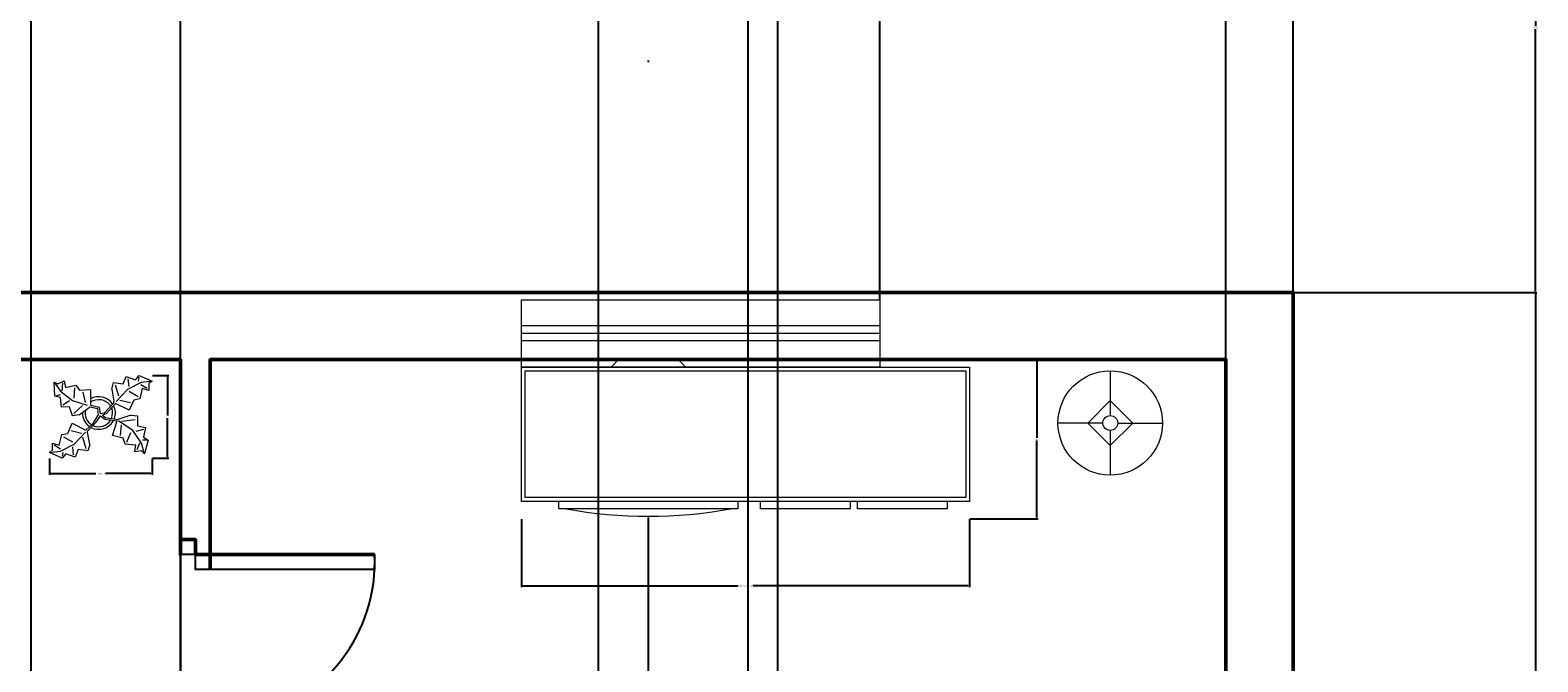
# Model space of a CAD drawing. Units: inches. Extents: x 821 to 2399, y 74 to 823.
# Tile 7 of 13: x 1128 to 1330, y 549 to 634. Entities that reach past the tile are written whole.
import ezdxf

# ---------------------------------------------------------------- set-up
doc = ezdxf.new("R2010")
doc.units = ezdxf.units.IN
doc.header["$MEASUREMENT"] = 0
doc.layers.get('0').update_dxf_attribs({"lineweight": 53})
for name, color, linetype, lineweight in [('A-ANNO-DIMS', 2, 'Continuous', 18), ('A-DOOR', 4, 'Continuous', 25), ('A-FURN', 8, 'Continuous', 18), ('A-GLAZ', 4, 'Continuous', 18), ('WALLS', 7, 'Continuous', 50)]:
    doc.layers.add(name, color=color, linetype=linetype, lineweight=lineweight)
doc.styles.get("Standard").update_dxf_attribs({"font": 'arial.ttf'})
doc.dimstyles.get("Standard").update_dxf_attribs({"dimtxt": 0.18, "dimasz": 0.18, "dimexe": 0.18, "dimexo": 0.0625, "dimgap": 0.09, "dimtad": 0, "dimtih": 1, "dimtoh": 1, "dimdec": 4, "dimzin": 0, "dimdsep": 46, "dimtxsty": 'Standard', "dimcen": 0.09, "dimadec": 0, "dimazin": 0, "dimtfac": 1, "dimtdec": 4, "dimtofl": 0, "dimtmove": 0, "dimatfit": 3, "dimfxl": 1, "dimtolj": 1, "dimtzin": 0, "dimarcsym": 0})

# ---------------------------------------------------------------- blocks, each defined once
blk = doc.blocks.new('Entertainment Center')
for p, q in [((-4, 0), (-5, -1)), ((4, 0), (-4, 0)), ((5, -1), (4, 0)), ((-17, -19), (-17, -1)), ((-17, -1), (43, -1)), ((-16.5, -18.5), (-16.5, -1.5)), ((-16.5, -1.5), (42.5, -1.5)), ((42.5, -1.5), (42.5, -18.5)), ((43, -1), (43, -19)), ((43, -19), (-17, -19)), ((42.5, -18.5), (-16.5, -18.5)), ((-12, -20), (-12, -19)), ((12, -20), (-12, -20)), ((12, -19), (12, -20)), ((15, -20), (15, -19)), ((27, -20), (15, -20)), ((27, -19), (27, -20)), ((28, -20), (28, -19)), ((40, -20), (28, -20)), ((40, -19), (40, -20))]:
    blk.add_line(p, q)
blk.add_arc((0, 40), 61, 259.6111, 280.3889)
blk = doc.blocks.new('Lamp - Table')
for p, q in [((0, 7), (0, 1)), ((0, 3), (-3, 0)), ((3, 0), (0, 3)), ((-1, 0), (-7, 0)), ((-3, 0), (0, -3)), ((0, -3), (3, 0)), ((1, 0), (7, 0)), ((0, -1), (0, -7))]:
    blk.add_line(p, q)
for radius in [7, 1]:
    blk.add_circle((0, 0), radius)
blk = doc.blocks.new('Plant - Rubber or Philodendron')
for p, q in [((-16.2005, 11.4774), (-13.9899, 8.1064)), ((-16.2005, 11.4774), (-14.8639, 10.7964)), ((-16.0159, 6.3329), (-16.2005, 11.4774)), ((-14.8639, 10.7964), (-12.6195, 11.8975)), ((-13.3174, 8.325), (-13.0735, 11.0065)), ((-12.6195, 11.8975), (-12.1909, 9.4345)), ((4.6914, 8.8812), (5.3859, 11.2828)), ((5.3859, 11.2828), (8.8871, 10.7908)), ((8.8871, 10.7908), (9.9809, 13.4933)), ((9.9809, 13.4933), (13.3837, 12.301)), ((15.3859, 11.3055), (10.3916, 8.7942)), ((10.5828, 12.6946), (10.8893, 9.7953)), ((13.3837, 12.301), (14.68, 13.9039)), ((14.5816, 13.2037), (14.3848, 11.8033)), ((14.68, 13.9039), (19.3848, 11.8146)), ((19.3848, 11.8146), (15.3859, 11.3055)), ((19.3848, 11.8146), (18.1868, 10.9119)), ((-14.0069, 5.8704), (-16.0159, 6.3329)), ((-15.3434, 6.5514), (-13.9984, 6.9884)), ((-13.5868, 2.2894), (-14.0069, 5.8704)), ((-13.9899, 8.1064), (-9.5434, 4.7185)), ((-12.1909, 9.4345), (-8.3829, 10.3)), ((-8.8369, 9.409), (-9.0894, 5.6095)), ((-8.3829, 10.3), (-7.0549, 8.501)), ((-7.0549, 8.501), (-3.0284, 8.6941)), ((-4.8529, 4.012), (-5.7184, 7.82)), ((-3.0284, 8.6941), (-3.0709, 3.1041)), ((4.6914, 8.8812), (5.5014, 4.4831)), ((5.9878, 10.4842), (7.1971, 6.3869)), ((10.3916, 8.7942), (6.2847, 4.4028)), ((14.2977, 6.1031), (10.9934, 7.9956)), ((15.7909, 9.1065), (14.8995, 5.3044)), ((15.2875, 10.6053), (17.5907, 9.2105)), ((18.1925, 8.4119), (15.7909, 9.1065)), ((18.1868, 10.9119), (18.1925, 8.4119)), ((-10.6784, 2.491), (-13.5868, 2.2894)), ((-13.1329, 3.1804), (-10.6614, 4.727)), ((-9.5858, -0.8715), (-10.6784, 2.491)), ((-9.5434, 4.7185), (-4.1917, 2.9888)), ((-9.1318, 0.0195), (-5.9793, 2.9025)), ((-7.1228, -0.443), (-3.5248, 2.2131)), ((-3.5248, 2.2131), (-3.3011, 2.4355)), ((-3.3011, 2.4355), (-0.5306, 1.7947)), ((-3.0709, 3.1041), (0.0797, 2.3163)), ((-0.5306, 1.7947), (-0.2255, -0.5527)), ((-0.5306, 1.7947), (-0.5306, 1.7947)), ((0.0797, 2.3163), (0.4866, -0.031)), ((0.4866, -0.031), (2.1141, 0.2298)), ((2.1141, 0.2298), (5.4346, 3.9146)), ((6.1032, 3.6844), (2.8262, -0.031)), ((5.4346, 3.9146), (5.5014, 4.4831)), ((11.1089, 1.1958), (6.1032, 3.6844)), ((7.7005, 4.8881), (11.5025, 3.9967)), ((12.7005, 4.8994), (11.1089, 1.1958)), ((14.8995, 5.3044), (12.7005, 4.8994)), ((-11.3237, -7.2629), (-9.7321, -3.5593)), ((-9.7321, -3.5593), (-4.7264, -6.0479)), ((-7.1228, -0.443), (-9.5858, -0.8715)), ((-2.019, -3.6148), (-4.7264, -6.0479)), ((-4.0579, -6.2781), (-0.9375, -3.1608)), ((-2.019, -3.6148), (-0.2255, -0.5527)), ((-0.9375, -3.1608), (0.5883, -0.8135)), ((0.5883, -0.8135), (2.2447, -2.0916)), ((2.8262, -0.031), (1.3003, -0.5527)), ((1.3003, -0.5527), (2.4193, -1.4655)), ((2.2447, -2.0916), (6.7108, -2.6626)), ((2.4193, -1.4655), (6.895, -2.1175)), ((4.943, -7.9659), (6.7108, -2.6626)), ((11.6605, -0.5413), (6.895, -2.1175)), ((12.3677, -6.1981), (7.219, -2.6772)), ((8.125, -4.0768), (7.7715, -7.9659)), ((8.3544, -2.7453), (13.1973, -2.1704)), ((11.6605, -0.5413), (14.1354, -0.8948)), ((14.1354, -0.8948), (14.1354, -4.4304)), ((14.1354, -4.4304), (16.9638, -5.1375)), ((16.9638, -5.1375), (16.2567, -8.673)), ((-16.8157, -10.7754), (-14.4141, -11.4699)), ((-16.8101, -13.2754), (-16.8157, -10.7754)), ((-14.4141, -11.4699), (-13.5228, -7.6679)), ((-13.5228, -7.6679), (-11.3237, -7.2629)), ((-12.921, -8.4665), (-9.6166, -10.359)), ((-6.3237, -7.2516), (-10.1257, -6.3602)), ((-9.0148, -11.1577), (-4.9047, -6.8122)), ((-4.611, -12.8477), (-5.8203, -8.7504)), ((-4.1246, -6.8466), (-4.0579, -6.2781)), ((-3.3146, -11.2447), (-4.1246, -6.8466)), ((8.8321, -9.0266), (4.943, -7.9659)), ((9.5392, -11.1479), (8.8321, -9.0266)), ((10.2463, -10.4408), (11.6605, -6.9053)), ((15.5496, -10.7943), (12.3677, -6.1981)), ((16.2567, -5.8446), (13.4283, -6.5517)), ((14.8425, -10.7943), (13.7819, -13.2692)), ((16.6103, -14.6834), (15.5496, -10.7943)), ((17.3174, -9.7337), (15.9032, -9.7337)), ((16.2567, -8.673), (18.0245, -9.7337)), ((18.0245, -9.7337), (16.6103, -14.6834)), ((-18.008, -14.1781), (-16.8101, -13.2754)), ((-18.008, -14.1781), (-14.0091, -13.669)), ((-13.3032, -16.2674), (-18.008, -14.1781)), ((-13.9107, -12.9688), (-16.2139, -11.574)), ((-14.0091, -13.669), (-9.0148, -11.1577)), ((-12.0069, -14.6645), (-13.3032, -16.2674)), ((-13.2048, -15.5672), (-13.008, -14.1668)), ((-8.6042, -15.8568), (-12.0069, -14.6645)), ((-9.206, -15.0581), (-9.5126, -12.1588)), ((-7.5103, -13.1543), (-8.6042, -15.8568)), ((-4.0092, -13.6463), (-7.5103, -13.1543)), ((-3.3146, -11.2447), (-4.0092, -13.6463)), ((13.4283, -11.5015), (9.5392, -11.1479)), ((13.0748, -13.9763), (13.4283, -11.5015)), ((15.5496, -13.6228), (13.0748, -13.9763)), ((16.6103, -14.6834), (15.5496, -13.6228))]:
    blk.add_line(p, q)
for centre, radius, start, end in [((0, 0), 6.1275, 34.37569, 120.1028), ((0.0308, 0.1664), 6, 178.6147, 235.1169), ((0.0308, 0.1664), 5, 168.1647, 238.6725), ((-0.0601, -0.2075), 5.2461, 33.82192, 124.9414), ((-0.2664, 0.1682), 5.2775, 338.4094, 20.03007), ((-0.098, 0.1364), 6.1288, 341.2017, 26.09184), ((-0.0234, 0.3825), 6.1492, 242.5812, 331.2714), ((-0.1102, 0.4886), 5.2883, 247.3711, 327.472)]:
    blk.add_arc(centre, radius, start, end)
blk = doc.blocks.new('WIN-48IN')
for p, q in [((3.5, 48), (3.5, 0)), ((4.5, 48), (4.5, 0)), ((5.5, 48), (5.5, 0))]:
    blk.add_line(p, q)
blk.add_lwpolyline([(9, 0), (0, 0), (0, 48), (9, 48)], close=True)
blk = doc.blocks.new('*D48')
at = {"layer": 'A-ANNO-DIMS', "color": 0, "lineweight": -2, "transparency": 16777216}
for p, q in [((1194.03, 568.12), (1194.03, 559.01)), ((1254.03, 568.12), (1254.03, 559.01)), ((1194.21, 559.19), (1223.05, 559.19)), ((1253.85, 559.19), (1225, 559.19))]:
    blk.add_line(p, q, dxfattribs=at)
at = {"layer": 'A-ANNO-DIMS', "color": 0, "lineweight": 50, "transparency": 16777216}
for points in [[(1194.21, 559.22), (1194.21, 559.16), (1194.03, 559.19)], [(1253.85, 559.22), (1253.85, 559.16), (1254.03, 559.19)]]:
    blk.add_solid(points, dxfattribs=at)
at = {"layer": 'Defpoints', "color": 0, "lineweight": 50, "transparency": 16777216}
for p in [(1194.03, 568.19), (1254.03, 568.19), (1254.03, 559.19)]:
    blk.add_point(p, dxfattribs=at)
at = {"layer": 'A-ANNO-DIMS', "color": 0, "transparency": 16777216, "insert": (1224.03, 559.19), "char_height": 0.18, "attachment_point": 5}
blk.add_mtext('\\A1;MEDIA UNIT 60', dxfattribs=at)
blk = doc.blocks.new('*D49')
at = {"layer": 'A-ANNO-DIMS', "color": 0, "lineweight": -2, "transparency": 16777216}
for p, q in [((1254.09, 589.52), (1263.21, 589.52)), ((1263.03, 589.34), (1263.03, 579.03)), ((1263.03, 568.37), (1263.03, 578.67)), ((1254.09, 568.19), (1263.21, 568.19))]:
    blk.add_line(p, q, dxfattribs=at)
at = {"layer": 'A-ANNO-DIMS', "color": 0, "lineweight": 50, "transparency": 16777216}
for points in [[(1263, 589.34), (1263.06, 589.34), (1263.03, 589.52)], [(1263, 568.37), (1263.06, 568.37), (1263.03, 568.19)]]:
    blk.add_solid(points, dxfattribs=at)
at = {"layer": 'Defpoints', "color": 0, "lineweight": 50, "transparency": 16777216}
for p in [(1254.03, 589.52), (1263.03, 589.52), (1254.03, 568.19)]:
    blk.add_point(p, dxfattribs=at)
at = {"layer": 'A-ANNO-DIMS', "color": 0, "transparency": 16777216, "insert": (1263.03, 578.85), "char_height": 0.18, "attachment_point": 5}
blk.add_mtext('\\A1;21', dxfattribs=at)
blk = doc.blocks.new('*D52')
at = {"layer": 'A-ANNO-DIMS', "color": 0, "lineweight": -2, "transparency": 16777216}
for p, q in [((1130.82, 576.25), (1130.82, 574.07)), ((1144.57, 576.25), (1144.57, 574.07)), ((1131, 574.25), (1137.04, 574.25)), ((1144.39, 574.25), (1138.35, 574.25))]:
    blk.add_line(p, q, dxfattribs=at)
at = {"layer": 'A-ANNO-DIMS', "color": 0, "lineweight": 50, "transparency": 16777216}
for points in [[(1131, 574.28), (1131, 574.22), (1130.82, 574.25)], [(1144.39, 574.28), (1144.39, 574.22), (1144.57, 574.25)]]:
    blk.add_solid(points, dxfattribs=at)
at = {"layer": 'Defpoints', "color": 0, "lineweight": 50, "transparency": 16777216}
for p in [(1130.82, 576.31), (1144.57, 576.31), (1144.57, 574.25)]:
    blk.add_point(p, dxfattribs=at)
at = {"layer": 'A-ANNO-DIMS', "color": 0, "transparency": 16777216, "insert": (1137.7, 574.25), "char_height": 0.18, "attachment_point": 5}
blk.add_mtext('\\A1;PLANT 14', dxfattribs=at)
blk = doc.blocks.new('*D53')
at = {"layer": 'A-ANNO-DIMS', "color": 0, "lineweight": -2, "transparency": 16777216}
for p, q in [((1144.63, 587.4), (1146.81, 587.4)), ((1146.63, 587.22), (1146.63, 582.04)), ((1146.63, 576.49), (1146.63, 581.67)), ((1144.63, 576.31), (1146.81, 576.31))]:
    blk.add_line(p, q, dxfattribs=at)
at = {"layer": 'A-ANNO-DIMS', "color": 0, "lineweight": 50, "transparency": 16777216}
for points in [[(1146.6, 587.22), (1146.66, 587.22), (1146.63, 587.4)], [(1146.6, 576.49), (1146.66, 576.49), (1146.63, 576.31)]]:
    blk.add_solid(points, dxfattribs=at)
at = {"layer": 'Defpoints', "color": 0, "lineweight": 50, "transparency": 16777216}
for p in [(1144.57, 587.4), (1146.63, 587.4), (1144.57, 576.31)]:
    blk.add_point(p, dxfattribs=at)
at = {"layer": 'A-ANNO-DIMS', "color": 0, "transparency": 16777216, "insert": (1146.63, 581.86), "char_height": 0.18, "attachment_point": 5}
blk.add_mtext('\\A1;11', dxfattribs=at)
blk = doc.blocks.new('*D79')
at = {"layer": 'A-ANNO-DIMS', "color": 0, "lineweight": -2, "transparency": 16777216}
for p, q in [((1297.44, 598.52), (1330, 598.52)), ((1329.82, 598.34), (1329.82, 399.7)), ((1329.82, 200.7), (1329.82, 399.34)), ((1297.44, 200.52), (1330, 200.52))]:
    blk.add_line(p, q, dxfattribs=at)
at = {"layer": 'A-ANNO-DIMS', "color": 0, "lineweight": 50, "transparency": 16777216}
for points in [[(1329.79, 598.34), (1329.85, 598.34), (1329.82, 598.52)], [(1329.79, 200.7), (1329.85, 200.7), (1329.82, 200.52)]]:
    blk.add_solid(points, dxfattribs=at)
at = {"layer": 'Defpoints', "color": 0, "lineweight": 50, "transparency": 16777216}
for p in [(1297.37, 598.52), (1297.37, 200.52), (1329.82, 200.52)]:
    blk.add_point(p, dxfattribs=at)
at = {"layer": 'A-ANNO-DIMS', "color": 0, "transparency": 16777216, "insert": (1329.82, 399.52), "char_height": 0.18, "attachment_point": 5}
blk.add_mtext('\\A1;398', dxfattribs=at)
blk = doc.blocks.new('*D87')
at = {"layer": 'A-ANNO-DIMS', "color": 0, "lineweight": -2, "transparency": 16777216}
for p, q in [((1122.09, 669.47), (1330, 669.47)), ((1329.82, 669.29), (1329.82, 634.18)), ((1329.82, 598.7), (1329.82, 633.81)), ((1122.09, 598.52), (1330, 598.52))]:
    blk.add_line(p, q, dxfattribs=at)
at = {"layer": 'A-ANNO-DIMS', "color": 0, "lineweight": 50, "transparency": 16777216}
for points in [[(1329.79, 669.29), (1329.85, 669.29), (1329.82, 669.47)], [(1329.79, 598.7), (1329.85, 598.7), (1329.82, 598.52)]]:
    blk.add_solid(points, dxfattribs=at)
at = {"layer": 'Defpoints', "color": 0, "lineweight": 50, "transparency": 16777216}
for p in [(1122.03, 669.47), (1122.03, 598.52), (1329.82, 598.52)]:
    blk.add_point(p, dxfattribs=at)
at = {"layer": 'A-ANNO-DIMS', "color": 0, "transparency": 16777216, "insert": (1329.82, 634), "char_height": 0.18, "attachment_point": 5}
blk.add_mtext('\\A1;70.95', dxfattribs=at)
blk = doc.blocks.new('*D92')
at = {"layer": 'A-ANNO-DIMS', "color": 0, "lineweight": -2, "transparency": 16777216}
for p, q in [((1128.37, 209.58), (1128.37, 786.75)), ((1128.55, 786.57), (1138.15, 786.57)), ((1148.19, 786.57), (1138.59, 786.57)), ((1148.37, 209.58), (1148.37, 786.75))]:
    blk.add_line(p, q, dxfattribs=at)
at = {"layer": 'A-ANNO-DIMS', "color": 0, "lineweight": 50, "transparency": 16777216}
for points in [[(1128.55, 786.6), (1128.55, 786.54), (1128.37, 786.57)], [(1148.19, 786.6), (1148.19, 786.54), (1148.37, 786.57)]]:
    blk.add_solid(points, dxfattribs=at)
at = {"layer": 'Defpoints', "color": 0, "lineweight": 50, "transparency": 16777216}
for p in [(1148.37, 786.57), (1128.37, 209.52), (1148.37, 209.52)]:
    blk.add_point(p, dxfattribs=at)
at = {"layer": 'A-ANNO-DIMS', "color": 0, "transparency": 16777216, "insert": (1138.37, 786.57), "char_height": 0.18, "attachment_point": 5}
blk.add_mtext('\\A1;20', dxfattribs=at)
blk = doc.blocks.new('*D94')
at = {"layer": 'A-ANNO-DIMS', "color": 0, "lineweight": -2, "transparency": 16777216}
for p, q in [((1204.37, 396.58), (1204.37, 786.75)), ((1204.55, 786.57), (1214.15, 786.57)), ((1224.19, 786.57), (1214.59, 786.57)), ((1224.37, 396.58), (1224.37, 786.75))]:
    blk.add_line(p, q, dxfattribs=at)
at = {"layer": 'A-ANNO-DIMS', "color": 0, "lineweight": 50, "transparency": 16777216}
for points in [[(1204.55, 786.6), (1204.55, 786.54), (1204.37, 786.57)], [(1224.19, 786.6), (1224.19, 786.54), (1224.37, 786.57)]]:
    blk.add_solid(points, dxfattribs=at)
at = {"layer": 'Defpoints', "color": 0, "lineweight": 50, "transparency": 16777216}
for p in [(1224.37, 786.57), (1204.37, 396.52), (1224.37, 396.52)]:
    blk.add_point(p, dxfattribs=at)
at = {"layer": 'A-ANNO-DIMS', "color": 0, "transparency": 16777216, "insert": (1214.37, 786.57), "char_height": 0.18, "attachment_point": 5}
blk.add_mtext('\\A1;20', dxfattribs=at)
blk = doc.blocks.new('*D95')
at = {"layer": 'A-ANNO-DIMS', "color": 0, "lineweight": -2, "transparency": 16777216}
for p, q in [((1228.37, 396.58), (1228.37, 786.75)), ((1228.55, 786.57), (1258.15, 786.57)), ((1288.19, 786.57), (1258.59, 786.57)), ((1288.37, 396.58), (1288.37, 786.75))]:
    blk.add_line(p, q, dxfattribs=at)
at = {"layer": 'A-ANNO-DIMS', "color": 0, "lineweight": 50, "transparency": 16777216}
for points in [[(1228.55, 786.6), (1228.55, 786.54), (1228.37, 786.57)], [(1288.19, 786.6), (1288.19, 786.54), (1288.37, 786.57)]]:
    blk.add_solid(points, dxfattribs=at)
at = {"layer": 'Defpoints', "color": 0, "lineweight": 50, "transparency": 16777216}
for p in [(1288.37, 786.57), (1228.37, 396.52), (1288.37, 396.52)]:
    blk.add_point(p, dxfattribs=at)
at = {"layer": 'A-ANNO-DIMS', "color": 0, "transparency": 16777216, "insert": (1258.37, 786.57), "char_height": 0.18, "attachment_point": 5}
blk.add_mtext('\\A1;60', dxfattribs=at)
blk = doc.blocks.new('*D98')
at = {"layer": 'A-ANNO-DIMS', "color": 0, "lineweight": -2, "transparency": 16777216}
for p, q in [((1242.03, 597.58), (1242.03, 786.75)), ((1242.21, 786.57), (1269.31, 786.57)), ((1297.19, 786.57), (1270.09, 786.57)), ((1297.37, 598.58), (1297.37, 786.75))]:
    blk.add_line(p, q, dxfattribs=at)
at = {"layer": 'A-ANNO-DIMS', "color": 0, "lineweight": 50, "transparency": 16777216}
for points in [[(1242.21, 786.6), (1242.21, 786.54), (1242.03, 786.57)], [(1297.19, 786.6), (1297.19, 786.54), (1297.37, 786.57)]]:
    blk.add_solid(points, dxfattribs=at)
at = {"layer": 'Defpoints', "color": 0, "lineweight": 50, "transparency": 16777216}
for p in [(1297.37, 786.57), (1297.37, 598.52), (1242.03, 597.52)]:
    blk.add_point(p, dxfattribs=at)
at = {"layer": 'A-ANNO-DIMS', "color": 0, "transparency": 16777216, "insert": (1269.7, 786.57), "char_height": 0.18, "attachment_point": 5}
blk.add_mtext('\\A1;55.35', dxfattribs=at)
blk = doc.blocks.new('*D138')
at = {"layer": 'A-ANNO-DIMS', "color": 0, "lineweight": -2, "transparency": 16777216}
for p, q in [((1210.94, 629.52), (1211.12, 629.52)), ((1211.03, 629.43), (1211.03, 629.61)), ((1211.03, 531.92), (1211.03, 568.34)), ((1211.21, 531.92), (1211.03, 531.92))]:
    blk.add_line(p, q, dxfattribs=at)
at = {"layer": 'A-ANNO-DIMS', "color": 0, "lineweight": 50, "transparency": 16777216}
blk.add_solid([(1211.06, 568.34), (1211, 568.34), (1211.03, 568.52)], dxfattribs=at)
at = {"layer": 'Defpoints', "color": 0, "lineweight": 50, "transparency": 16777216}
for p in [(1211.03, 629.52), (1211.03, 568.52)]:
    blk.add_point(p, dxfattribs=at)
at = {"layer": 'A-ANNO-DIMS', "color": 0, "transparency": 16777216, "insert": (1211.5, 531.92), "char_height": 0.18, "attachment_point": 5}
blk.add_mtext('\\A1;R61', dxfattribs=at)

msp = doc.modelspace()

# ---------------------------------------------------------------- linework, layer by layer
at = {"layer": 'A-DOOR'}
msp.add_lwpolyline([(1174.3735, 519.3933), (1174.3735, 521.3933), (1150.3735, 521.3933), (1150.3735, 519.3933), (1174.3735, 519.3933, 0.36630785), (1157.4504, 541.3933, 0.36630785), (1174.3735, 563.3933), (1174.3735, 561.3933), (1150.3735, 561.3933), (1150.3735, 563.3933), (1148.3735, 563.3933), (1148.3735, 519.3933), (1150.3735, 519.3933), (1150.3735, 517.3933), (1148.3735, 517.3933), (1148.3735, 519.3933), (1148.3735, 465.5195)], format="xyb", dxfattribs=at)
at = {"layer": 'WALLS'}
msp.add_lwpolyline([(1050.641, 200.5195), (1050.641, 170.9407), (1121.9086, 170.9407), (1128.124, 170.9407), (1050.641, 170.9407), (1050.641, 106.8645), (1128.124, 106.8645), (1128.124, 170.9407), (1128.124, 200.5195), (1288.3735, 200.5195), (1297.3735, 200.5195), (1297.3735, 598.5195), (853.3735, 598.5195), (853.3735, 292.549), (922.3673, 292.5195), (1043.3735, 292.5195), (1043.3735, 209.5195), (1043.3735, 200.5195)], close=True, dxfattribs=at)
for points in [[(862.3735, 589.5195), (1148.3735, 589.5195), (1148.3735, 563.3933), (1148.3735, 565.3933), (1150.3735, 565.3933), (1150.3735, 563.3933), (1174.3735, 563.3933)], [(1152.3735, 521.3933), (1152.3735, 469.5195), (1288.3735, 469.5195), (1288.3735, 589.5195), (1152.3735, 589.5195), (1152.3735, 561.3933)]]:
    msp.add_lwpolyline(points, dxfattribs=at)

# ---------------------------------------------------------------- block references
at = {"layer": 'A-FURN'}
for name, p in [('Entertainment Center', (1211.0276, 589.5195)), ('Lamp - Table', (1272.8779, 581.0195))]:
    msp.add_blockref(name, p, dxfattribs=at)
at = {"layer": 'A-FURN', "xscale": 0.367734597948145, "yscale": 0.367734597948145, "zscale": 0.367734597948145}
msp.add_blockref('Plant - Rubber or Philodendron', (1137.443, 582.2899), dxfattribs=at)
at = {"layer": 'A-GLAZ', "rotation": 269.9999999999985}
msp.add_blockref('WIN-48IN', (1194.0274, 597.5199), dxfattribs=at)

# ---------------------------------------------------------------- dimensions: what is measured, and where the dimension line sits
at = {"layer": 'A-ANNO-DIMS'}
for base, p1, p2, override, picture, middle in [((1148.3735, 786.5664), (1128.3735, 209.5195), (1148.3735, 209.5195), {"dimdec": 0, "dimlfac": 1, "dimrnd": 0, "dimzin": 0, "dimdsep": 46, "dimlunit": 2}, '*D92', (1138.3735, 786.5664)), ((1224.3735, 786.5664), (1204.3735, 396.5195), (1224.3735, 396.5195), {"dimdec": 0, "dimlfac": 1, "dimrnd": 0, "dimzin": 0, "dimdsep": 46, "dimlunit": 2}, '*D94', (1214.3735, 786.5664)), ((1288.3735, 786.5664), (1228.3735, 396.5195), (1288.3735, 396.5195), {"dimdec": 0, "dimlfac": 1, "dimrnd": 0, "dimzin": 0, "dimdsep": 46, "dimlunit": 2}, '*D95', (1258.3735, 786.5664)), ((1297.3735, 786.5664), (1242.0276, 597.5195), (1297.3735, 598.5195), {"dimdec": 2, "dimlfac": 1, "dimrnd": 0, "dimzin": 0, "dimdsep": 46, "dimlunit": 2}, '*D98', (1269.7005, 786.5664))]:
    dim = msp.add_linear_dim(base=base, p1=p1, p2=p2, dimstyle='Standard', override=override, dxfattribs=at)
    dim.commit()
    dim.dimension.update_dxf_attribs({"geometry": picture, "text_midpoint": middle})
for base, p1, p2, override, picture, middle in [((1329.8235, 598.5195), (1122.0283, 669.4726), (1122.0283, 598.5195), {"dimdec": 2, "dimlfac": 1, "dimrnd": 0, "dimzin": 0, "dimdsep": 46, "dimlunit": 2}, '*D87', (1329.8235, 633.996)), ((1329.8235, 200.5195), (1297.3735, 598.5195), (1297.3735, 200.5195), {"dimdec": 0, "dimlfac": 1, "dimrnd": 0, "dimzin": 0, "dimdsep": 46, "dimlunit": 2}, '*D79', (1329.8235, 399.5195)), ((1263.0276, 589.5195), (1254.0276, 568.1861), (1254.0276, 589.5195), {"dimdec": 0, "dimlfac": 1, "dimrnd": 0, "dimzin": 0, "dimdsep": 46, "dimlunit": 2}, '*D49', (1263.0276, 578.8528)), ((1146.6341, 587.4028), (1144.5715, 576.3078), (1144.5715, 587.4028), {"dimdec": 0, "dimlfac": 1, "dimrnd": 0, "dimzin": 0, "dimdsep": 46, "dimlunit": 2}, '*D53', (1146.6341, 581.8553))]:
    dim = msp.add_linear_dim(base=base, p1=p1, p2=p2, angle=90, dimstyle='Standard', override=override, dxfattribs=at)
    dim.commit()
    dim.dimension.update_dxf_attribs({"geometry": picture, "text_midpoint": middle})
dim = msp.add_radius_dim(center=(1211.0276, 629.5195), mpoint=(1211.028, 568.5195), dimstyle='Standard', override={"dimdec": 0, "dimlfac": 1, "dimrnd": 0, "dimzin": 0, "dimdsep": 46, "dimlunit": 2}, dxfattribs=at)
dim.commit()
dim.dimension.update_dxf_attribs({"geometry": '*D138', "text_midpoint": (1211.4959, 531.9195), "dimtype": 164})
for base, p1, p2, text, picture, middle in [((1144.5715, 574.2452), (1130.8208, 576.3078), (1144.5715, 576.3078), 'PLANT <>', '*D52', (1137.6961, 574.2452)), ((1254.0276, 559.1861), (1194.0276, 568.1861), (1254.0276, 568.1861), 'MEDIA UNIT <>', '*D48', (1224.0276, 559.1861))]:
    dim = msp.add_linear_dim(base=base, p1=p1, p2=p2, text=text, dimstyle='Standard', override={"dimdec": 0, "dimlfac": 1, "dimrnd": 0, "dimzin": 0, "dimdsep": 46, "dimlunit": 2}, dxfattribs=at)
    dim.commit()
    dim.dimension.update_dxf_attribs({"geometry": picture, "text_midpoint": middle})

doc.saveas('drawing.dxf')
